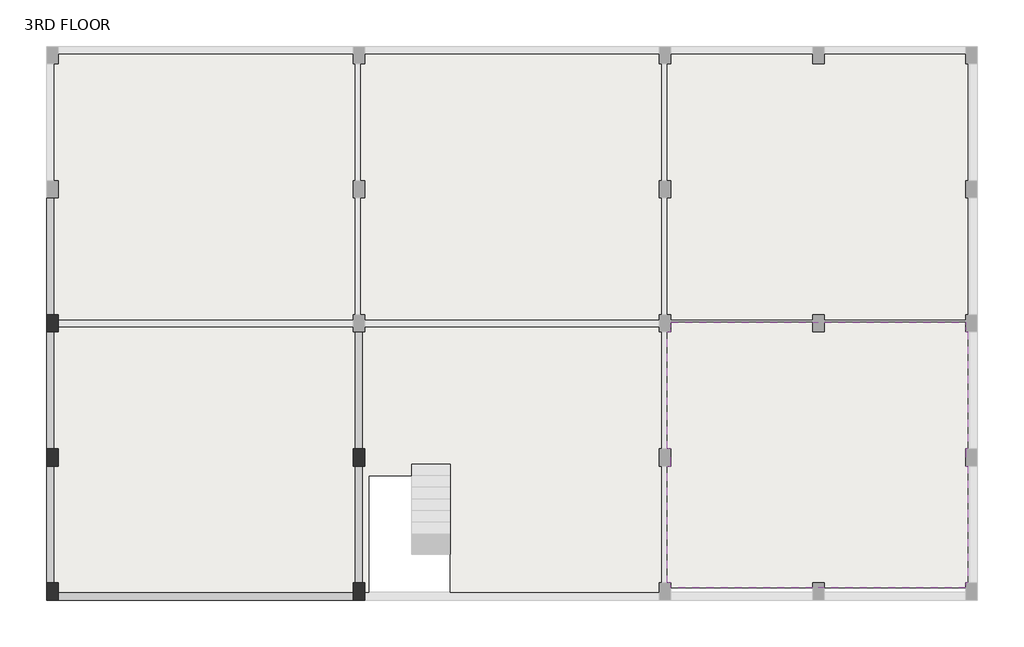
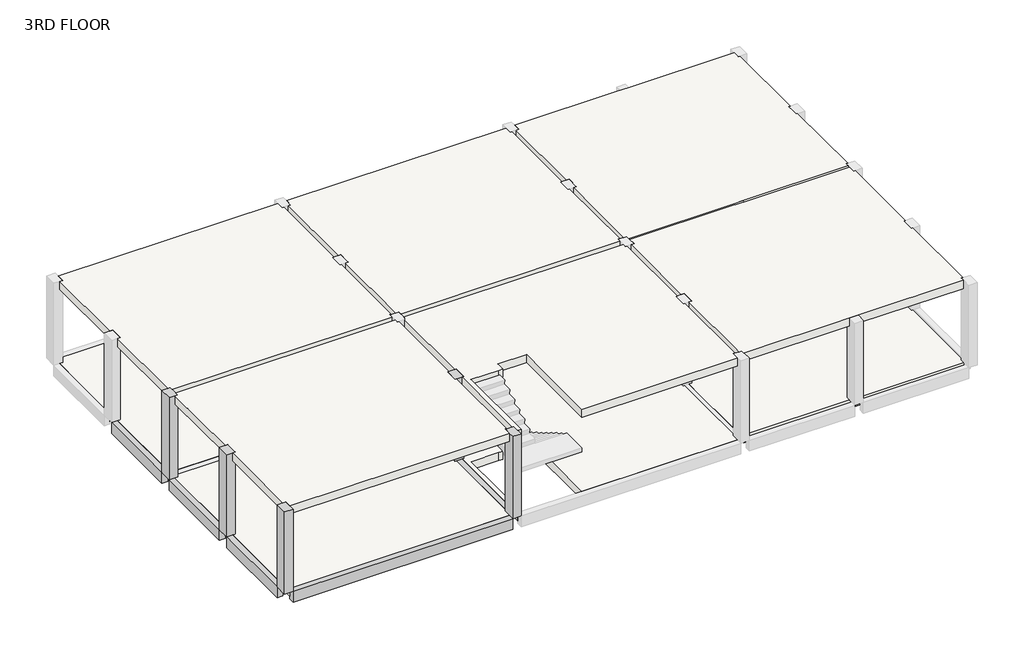
# One storey, part 1 of 2: 6 beams, 5 columns, 2 slabs.
"""IFC4 building model written with IfcOpenShell, lengths in millimetres."""

from ifc_helpers import new_model, si_unit, origin, place, context, project, spatial, faceted_brep, element, save

model = new_model("IFC4")

# Units and contexts
model_context = context("Model", 3, world=origin())
ifc_project = project(units=[si_unit("LENGTHUNIT", "METRE", prefix="MILLI")], contexts=[model_context])

# Site, building, storey
site = spatial("IfcSite", under=ifc_project)
building = spatial("IfcBuilding", under=site)
storey = spatial("IfcBuildingStorey", under=building, Name="3RD FLOOR", Elevation=9144.0)

# Beams
placement = place(None, origin())
element("IfcBeam", 1, ObjectType="M_Concrete-Rectangular Beam : 200MMX400MM", at=placement, inside=storey, context=model_context, shape_type="Brep", body=[
    faceted_brep([(-11680.6874017, 1747.7008557, 9144.0), (-11680.6874017, 1547.7008557, 9144.0), (-3980.6874017, 1547.7008557, 9144.0), (-3980.6874017, 1747.7008557, 9144.0), (-11680.6874017, 1747.7008557, 8744.0), (-11680.6874017, 1747.7008557, 8844.0), (-3980.6874017, 1747.7008557, 8844.0), (-3980.6874017, 1747.7008557, 8744.0), (-11680.6874017, 1547.7008557, 8744.0), (-3980.6874017, 1547.7008557, 8744.0)], [[[0, 1, 2, 3]], [[4, 5, 0, 3, 6, 7]], [[8, 4, 7, 9]], [[1, 8, 9, 2]], [[1, 0, 5, 4, 8]], [[2, 9, 7, 6, 3]]]),
])
element("IfcBeam", 2, ObjectType="M_Concrete-Rectangular Beam : 200MMX400MM", at=placement, inside=storey, context=model_context, shape_type="Brep", body=[
    faceted_brep([(-11980.6874017, 8997.7008557, 9144.0), (-11780.6874017, 8997.7008557, 9144.0), (-11780.6874017, 12047.7008557, 9144.0), (-11980.6874017, 12047.7008557, 9144.0), (-11980.6874017, 8997.7008557, 8744.0), (-11980.6874017, 12047.7008557, 8744.0), (-11780.6874017, 8997.7008557, 8744.0), (-11780.6874017, 12047.7008557, 8744.0), (-11780.6874017, 8997.7008557, 8844.0), (-11780.6874017, 12047.7008557, 8844.0)], [[[0, 1, 2, 3]], [[4, 0, 3, 5]], [[6, 4, 5, 7]], [[1, 8, 6, 7, 9, 2]], [[1, 0, 4, 6, 8]], [[2, 9, 7, 5, 3]]]),
])
element("IfcBeam", 3, ObjectType="M_Concrete-Rectangular Beam : 200MMX400MM", at=placement, inside=storey, context=model_context, shape_type="Brep", body=[
    faceted_brep([(-11980.6874017, 5497.7008557, 9144.0), (-11780.6874017, 5497.7008557, 9144.0), (-11780.6874017, 8547.7008557, 9144.0), (-11980.6874017, 8547.7008557, 9144.0), (-11980.6874017, 5497.7008557, 8744.0), (-11980.6874017, 8547.7008557, 8744.0), (-11780.6874017, 5497.7008557, 8744.0), (-11780.6874017, 8547.7008557, 8744.0), (-11780.6874017, 5497.7008557, 8844.0), (-11780.6874017, 8547.7008557, 8844.0)], [[[0, 1, 2, 3]], [[4, 0, 3, 5]], [[6, 4, 5, 7]], [[1, 8, 6, 7, 9, 2]], [[2, 9, 7, 5, 3]], [[1, 0, 4, 6, 8]]]),
])
element("IfcBeam", 4, ObjectType="M_Concrete-Rectangular Beam : 200MMX400MM", at=placement, inside=storey, context=model_context, shape_type="Brep", body=[
    faceted_brep([(-11980.6874017, 1997.7008557, 9144.0), (-11780.6874017, 1997.7008557, 9144.0), (-11780.6874017, 5047.7008557, 9144.0), (-11980.6874017, 5047.7008557, 9144.0), (-11980.6874017, 1997.7008557, 8744.0), (-11980.6874017, 5047.7008557, 8744.0), (-11780.6874017, 1997.7008557, 8744.0), (-11780.6874017, 5047.7008557, 8744.0), (-11780.6874017, 1997.7008557, 8844.0), (-11780.6874017, 5047.7008557, 8844.0)], [[[0, 1, 2, 3]], [[4, 0, 3, 5]], [[6, 4, 5, 7]], [[1, 8, 6, 7, 9, 2]], [[1, 0, 4, 6, 8]], [[2, 9, 7, 5, 3]]]),
])
element("IfcBeam", 5, ObjectType="M_Concrete-Rectangular Beam : 200MMX400MM", at=placement, inside=storey, context=model_context, shape_type="Brep", body=[
    faceted_brep([(-3930.6874017, 5047.7008557, 9144.0), (-3930.6874017, 1997.7008557, 9144.0), (-3730.6874017, 1997.7008557, 9144.0), (-3730.6874017, 5047.7008557, 9144.0), (-3730.6874017, 1997.7008557, 8844.0), (-3730.6874017, 1997.7008557, 8744.0), (-3730.6874017, 5047.7008557, 8744.0), (-3730.6874017, 5047.7008557, 8844.0), (-3930.6874017, 1997.7008557, 8744.0), (-3930.6874017, 5047.7008557, 8744.0), (-3930.6874017, 5047.7008557, 8844.0), (-3930.6874017, 1997.7008557, 8844.0)], [[[0, 1, 2, 3]], [[3, 2, 4, 5, 6, 7]], [[6, 5, 8, 9]], [[1, 0, 10, 9, 8, 11]], [[8, 5, 4, 2, 1, 11]], [[0, 3, 7, 6, 9, 10]]]),
])
element("IfcBeam", 6, ObjectType="M_Concrete-Rectangular Beam : 200MMX400MM", at=placement, inside=storey, context=model_context, shape_type="Brep", body=[
    faceted_brep([(-3930.6874017, 8547.7008557, 9144.0), (-3930.6874017, 5497.7008557, 9144.0), (-3730.6874017, 5497.7008557, 9144.0), (-3730.6874017, 8547.7008557, 9144.0), (-3730.6874017, 5497.7008557, 8844.0), (-3730.6874017, 5497.7008557, 8744.0), (-3730.6874017, 8547.7008557, 8744.0), (-3730.6874017, 8547.7008557, 8844.0), (-3930.6874017, 5497.7008557, 8744.0), (-3930.6874017, 8547.7008557, 8744.0), (-3930.6874017, 8547.7008557, 8844.0), (-3930.6874017, 5497.7008557, 8844.0)], [[[0, 1, 2, 3]], [[3, 2, 4, 5, 6, 7]], [[6, 5, 8, 9]], [[1, 0, 10, 9, 8, 11]], [[0, 3, 7, 6, 9, 10]], [[8, 5, 4, 2, 1, 11]]]),
])

# Columns
element("IfcColumn", 7, ObjectType="M_Concrete-Rectangular-Column : 300 x 450mm", at=placement, inside=storey, context=model_context, shape_type="Brep", body=[
    faceted_brep([(-11680.6874017, 8997.7008557, 9144.0), (-11680.6874017, 8547.7008557, 9144.0), (-11980.6874017, 8547.7008557, 9144.0), (-11980.6874017, 8997.7008557, 9144.0), (-11680.6874017, 8997.7008557, 11892.0), (-11680.6874017, 8997.7008557, 12192.0), (-11680.6874017, 8872.7008557, 12192.0), (-11680.6874017, 8672.7008557, 12192.0), (-11680.6874017, 8547.7008557, 12192.0), (-11680.6874017, 8547.7008557, 11892.0), (-11780.6874017, 8547.7008557, 12192.0), (-11980.6874017, 8547.7008557, 12192.0), (-11980.6874017, 8997.7008557, 12192.0), (-11780.6874017, 8997.7008557, 12192.0)], [[[0, 1, 2, 3]], [[1, 0, 4, 5, 6, 7, 8, 9]], [[2, 1, 9, 8, 10, 11]], [[3, 2, 11, 12]], [[0, 3, 12, 13, 5, 4]], [[12, 11, 10, 8, 7, 6, 5, 13]]]),
])
element("IfcColumn", 8, ObjectType="M_Concrete-Rectangular-Column : 300 x 450mm", at=placement, inside=storey, context=model_context, shape_type="Brep", body=[
    faceted_brep([(-11680.6874017, 1997.7008557, 9144.0), (-11680.6874017, 1547.7008557, 9144.0), (-11980.6874017, 1547.7008557, 9144.0), (-11980.6874017, 1997.7008557, 9144.0), (-11680.6874017, 1997.7008557, 11892.0), (-11680.6874017, 1997.7008557, 12192.0), (-11680.6874017, 1747.7008557, 12192.0), (-11680.6874017, 1547.7008557, 12192.0), (-11980.6874017, 1547.7008557, 12192.0), (-11980.6874017, 1997.7008557, 12192.0), (-11780.6874017, 1997.7008557, 12192.0)], [[[0, 1, 2, 3]], [[1, 0, 4, 5, 6, 7]], [[2, 1, 7, 8]], [[3, 2, 8, 9]], [[0, 3, 9, 10, 5, 4]], [[8, 7, 6, 5, 10, 9]]]),
])
element("IfcColumn", 9, ObjectType="M_Concrete-Rectangular-Column : 300 x 450mm", at=placement, inside=storey, context=model_context, shape_type="Brep", body=[
    faceted_brep([(-3680.6874017, 5497.7008557, 9144.0), (-3680.6874017, 5047.7008557, 9144.0), (-3980.6874017, 5047.7008557, 9144.0), (-3980.6874017, 5497.7008557, 9144.0), (-3680.6874017, 5497.7008557, 11892.0), (-3680.6874017, 5497.7008557, 12192.0), (-3680.6874017, 5047.7008557, 12192.0), (-3680.6874017, 5047.7008557, 11892.0), (-3730.6874017, 5047.7008557, 12192.0), (-3930.6874017, 5047.7008557, 12192.0), (-3980.6874017, 5047.7008557, 12192.0), (-3980.6874017, 5047.7008557, 11892.0), (-3980.6874017, 5497.7008557, 12192.0), (-3980.6874017, 5497.7008557, 11892.0), (-3930.6874017, 5497.7008557, 12192.0), (-3730.6874017, 5497.7008557, 12192.0)], [[[0, 1, 2, 3]], [[1, 0, 4, 5, 6, 7]], [[2, 1, 7, 6, 8, 9, 10, 11]], [[3, 2, 11, 10, 12, 13]], [[0, 3, 13, 12, 14, 15, 5, 4]], [[6, 5, 15, 14, 12, 10, 9, 8]]]),
])
element("IfcColumn", 10, ObjectType="M_Concrete-Rectangular-Column : 300 x 450mm", at=placement, inside=storey, context=model_context, shape_type="Brep", body=[
    faceted_brep([(-3680.6874017, 1997.7008557, 9144.0), (-3680.6874017, 1547.7008557, 9144.0), (-3980.6874017, 1547.7008557, 9144.0), (-3980.6874017, 1997.7008557, 9144.0), (-3680.6874017, 1997.7008557, 11892.0), (-3680.6874017, 1997.7008557, 12192.0), (-3680.6874017, 1747.7008557, 12192.0), (-3680.6874017, 1547.7008557, 12192.0), (-3980.6874017, 1547.7008557, 12192.0), (-3980.6874017, 1747.7008557, 12192.0), (-3980.6874017, 1997.7008557, 12192.0), (-3980.6874017, 1997.7008557, 11892.0), (-3930.6874017, 1997.7008557, 12192.0), (-3730.6874017, 1997.7008557, 12192.0)], [[[0, 1, 2, 3]], [[1, 0, 4, 5, 6, 7]], [[2, 1, 7, 8]], [[3, 2, 8, 9, 10, 11]], [[0, 3, 11, 10, 12, 13, 5, 4]], [[8, 7, 6, 5, 13, 12, 10, 9]]]),
])
element("IfcColumn", 11, ObjectType="M_Concrete-Rectangular-Column : 300 x 450mm", at=placement, inside=storey, context=model_context, shape_type="Brep", body=[
    faceted_brep([(-11680.6874017, 5497.7008557, 9144.0), (-11680.6874017, 5047.7008557, 9144.0), (-11980.6874017, 5047.7008557, 9144.0), (-11980.6874017, 5497.7008557, 9144.0), (-11680.6874017, 5497.7008557, 11892.0), (-11680.6874017, 5497.7008557, 12192.0), (-11680.6874017, 5047.7008557, 12192.0), (-11680.6874017, 5047.7008557, 11892.0), (-11780.6874017, 5047.7008557, 12192.0), (-11980.6874017, 5047.7008557, 12192.0), (-11980.6874017, 5497.7008557, 12192.0), (-11780.6874017, 5497.7008557, 12192.0)], [[[0, 1, 2, 3]], [[1, 0, 4, 5, 6, 7]], [[2, 1, 7, 6, 8, 9]], [[3, 2, 9, 10]], [[0, 3, 10, 11, 5, 4]], [[6, 5, 11, 10, 9, 8]]]),
])

# Slabs
element("IfcSlab", 12, ObjectType="Generic 300mm", at=placement, inside=storey, context=model_context, shape_type="Brep", body=[
    faceted_brep([(-11680.6874017, 15547.7008557, 8844.0), (-11680.6874017, 15797.7008557, 8844.0), (-3980.6874017, 15797.7008557, 8844.0), (-3980.6874017, 15547.7008557, 8844.0), (-3930.6874017, 15547.7008557, 8844.0), (-3930.6874017, 12497.7008557, 8844.0), (-3980.6874017, 12497.7008557, 8844.0), (-3980.6874017, 12047.7008557, 8844.0), (-3930.6874017, 12047.7008557, 8844.0), (-3930.6874017, 8997.7008557, 8844.0), (-3980.6874017, 8997.7008557, 8844.0), (-3980.6874017, 8872.7008557, 8844.0), (-11680.6874017, 8872.7008557, 8844.0), (-11680.6874017, 8997.7008557, 8844.0), (-11780.6874017, 8997.7008557, 8844.0), (-11780.6874017, 12047.7008557, 8844.0), (-11680.6874017, 12047.7008557, 8844.0), (-11680.6874017, 12497.7008557, 8844.0), (-11780.6874017, 12497.7008557, 8844.0), (-11780.6874017, 15547.7008557, 8844.0), (-11680.6874017, 15797.7008557, 9144.0), (-11680.6874017, 15547.7008557, 9144.0), (-11780.6874017, 15547.7008557, 9144.0), (-11780.6874017, 12497.7008557, 9144.0), (-11680.6874017, 12497.7008557, 9144.0), (-11680.6874017, 12047.7008557, 9144.0), (-11780.6874017, 12047.7008557, 9144.0), (-11780.6874017, 8997.7008557, 9144.0), (-11680.6874017, 8997.7008557, 9144.0), (-11680.6874017, 8872.7008557, 9144.0), (-3980.6874017, 8872.7008557, 9144.0), (-3980.6874017, 8997.7008557, 9144.0), (-3930.6874017, 8997.7008557, 9144.0), (-3930.6874017, 12047.7008557, 9144.0), (-3980.6874017, 12047.7008557, 9144.0), (-3980.6874017, 12497.7008557, 9144.0), (-3930.6874017, 12497.7008557, 9144.0), (-3930.6874017, 15547.7008557, 9144.0), (-3980.6874017, 15547.7008557, 9144.0), (-3980.6874017, 15797.7008557, 9144.0)], [[[0, 1, 2, 3, 4, 5, 6, 7, 8, 9, 10, 11, 12, 13, 14, 15, 16, 17, 18, 19]], [[20, 21, 22, 23, 24, 25, 26, 27, 28, 29, 30, 31, 32, 33, 34, 35, 36, 37, 38, 39]], [[1, 0, 21, 20]], [[2, 1, 20, 39]], [[3, 2, 39, 38]], [[4, 3, 38, 37]], [[5, 4, 37, 36]], [[6, 5, 36, 35]], [[7, 6, 35, 34]], [[8, 7, 34, 33]], [[9, 8, 33, 32]], [[10, 9, 32, 31]], [[11, 10, 31, 30]], [[12, 11, 30, 29]], [[13, 12, 29, 28]], [[14, 13, 28, 27]], [[15, 14, 27, 26]], [[16, 15, 26, 25]], [[17, 16, 25, 24]], [[18, 17, 24, 23]], [[19, 18, 23, 22]], [[0, 19, 22, 21]]]),
    faceted_brep([(-3680.6874017, 15547.7008557, 8844.0), (-3680.6874017, 15797.7008557, 8844.0), (4019.3125983, 15797.7008557, 8844.0), (4019.3125983, 15547.7008557, 8844.0), (4069.3125983, 15547.7008557, 8844.0), (4069.3125983, 12497.7008557, 8844.0), (4019.3125983, 12497.7008557, 8844.0), (4019.3125983, 12047.7008557, 8844.0), (4069.3125983, 12047.7008557, 8844.0), (4069.3125983, 8997.7008557, 8844.0), (4019.3125983, 8997.7008557, 8844.0), (4019.3125983, 8872.7008557, 8844.0), (-3680.6874017, 8872.7008557, 8844.0), (-3680.6874017, 8997.7008557, 8844.0), (-3730.6874017, 8997.7008557, 8844.0), (-3780.6874017, 8997.7008557, 8844.0), (-3780.6874017, 12047.7008557, 8844.0), (-3730.6874017, 12047.7008557, 8844.0), (-3680.6874017, 12047.7008557, 8844.0), (-3680.6874017, 12497.7008557, 8844.0), (-3730.6874017, 12497.7008557, 8844.0), (-3780.6874017, 12497.7008557, 8844.0), (-3780.6874017, 15547.7008557, 8844.0), (-3730.6874017, 15547.7008557, 8844.0), (-3680.6874017, 15797.7008557, 9144.0), (-3680.6874017, 15547.7008557, 9144.0), (-3780.6874017, 15547.7008557, 9144.0), (-3780.6874017, 12497.7008557, 9144.0), (-3680.6874017, 12497.7008557, 9144.0), (-3680.6874017, 12047.7008557, 9144.0), (-3780.6874017, 12047.7008557, 9144.0), (-3780.6874017, 8997.7008557, 9144.0), (-3680.6874017, 8997.7008557, 9144.0), (-3680.6874017, 8872.7008557, 9144.0), (4019.3125983, 8872.7008557, 9144.0), (4019.3125983, 8997.7008557, 9144.0), (4069.3125983, 8997.7008557, 9144.0), (4069.3125983, 12047.7008557, 9144.0), (4019.3125983, 12047.7008557, 9144.0), (4019.3125983, 12497.7008557, 9144.0), (4069.3125983, 12497.7008557, 9144.0), (4069.3125983, 15547.7008557, 9144.0), (4019.3125983, 15547.7008557, 9144.0), (4019.3125983, 15797.7008557, 9144.0)], [[[0, 1, 2, 3, 4, 5, 6, 7, 8, 9, 10, 11, 12, 13, 14, 15, 16, 17, 18, 19, 20, 21, 22, 23]], [[24, 25, 26, 27, 28, 29, 30, 31, 32, 33, 34, 35, 36, 37, 38, 39, 40, 41, 42, 43]], [[1, 0, 25, 24]], [[2, 1, 24, 43]], [[3, 2, 43, 42]], [[4, 3, 42, 41]], [[5, 4, 41, 40]], [[6, 5, 40, 39]], [[7, 6, 39, 38]], [[8, 7, 38, 37]], [[9, 8, 37, 36]], [[10, 9, 36, 35]], [[11, 10, 35, 34]], [[12, 11, 34, 33]], [[13, 12, 33, 32]], [[15, 14, 13, 32, 31]], [[16, 15, 31, 30]], [[18, 17, 16, 30, 29]], [[19, 18, 29, 28]], [[21, 20, 19, 28, 27]], [[22, 21, 27, 26]], [[0, 23, 22, 26, 25]]]),
    faceted_brep([(4319.3125983, 15547.7008557, 8844.0), (4319.3125983, 15797.7008557, 8844.0), (8019.3125983, 15797.7008557, 8844.0), (8319.3125983, 15797.7008557, 8844.0), (12019.3125983, 15797.7008557, 8844.0), (12019.3125983, 15547.7008557, 8844.0), (12069.3125983, 15547.7008557, 8844.0), (12069.3125983, 12497.7008557, 8844.0), (12019.3125983, 12497.7008557, 8844.0), (12019.3125983, 12047.7008557, 8844.0), (12069.3125983, 12047.7008557, 8844.0), (12069.3125983, 8997.7008557, 8844.0), (12019.3125983, 8997.7008557, 8844.0), (12019.3125983, 8872.7008557, 8844.0), (8319.3125983, 8872.7008557, 8844.0), (8019.3125983, 8872.7008557, 8844.0), (4319.3125983, 8872.7008557, 8844.0), (4319.3125983, 8997.7008557, 8844.0), (4269.3125983, 8997.7008557, 8844.0), (4219.3125983, 8997.7008557, 8844.0), (4219.3125983, 12047.7008557, 8844.0), (4269.3125983, 12047.7008557, 8844.0), (4319.3125983, 12047.7008557, 8844.0), (4319.3125983, 12497.7008557, 8844.0), (4269.3125983, 12497.7008557, 8844.0), (4219.3125983, 12497.7008557, 8844.0), (4219.3125983, 15547.7008557, 8844.0), (4269.3125983, 15547.7008557, 8844.0), (4319.3125983, 15797.7008557, 9144.0), (4319.3125983, 15547.7008557, 9144.0), (4219.3125983, 15547.7008557, 9144.0), (4219.3125983, 12497.7008557, 9144.0), (4319.3125983, 12497.7008557, 9144.0), (4319.3125983, 12047.7008557, 9144.0), (4219.3125983, 12047.7008557, 9144.0), (4219.3125983, 8997.7008557, 9144.0), (4319.3125983, 8997.7008557, 9144.0), (4319.3125983, 8872.7008557, 9144.0), (8019.3125983, 8872.7008557, 9144.0), (8319.3125983, 8872.7008557, 9144.0), (12019.3125983, 8872.7008557, 9144.0), (12019.3125983, 8997.7008557, 9144.0), (12069.3125983, 8997.7008557, 9144.0), (12069.3125983, 12047.7008557, 9144.0), (12019.3125983, 12047.7008557, 9144.0), (12019.3125983, 12497.7008557, 9144.0), (12069.3125983, 12497.7008557, 9144.0), (12069.3125983, 15547.7008557, 9144.0), (12019.3125983, 15547.7008557, 9144.0), (12019.3125983, 15797.7008557, 9144.0), (8319.3125983, 15797.7008557, 9144.0), (8019.3125983, 15797.7008557, 9144.0)], [[[0, 1, 2, 3, 4, 5, 6, 7, 8, 9, 10, 11, 12, 13, 14, 15, 16, 17, 18, 19, 20, 21, 22, 23, 24, 25, 26, 27]], [[28, 29, 30, 31, 32, 33, 34, 35, 36, 37, 38, 39, 40, 41, 42, 43, 44, 45, 46, 47, 48, 49, 50, 51]], [[1, 0, 29, 28]], [[4, 3, 2, 1, 28, 51, 50, 49]], [[5, 4, 49, 48]], [[6, 5, 48, 47]], [[7, 6, 47, 46]], [[8, 7, 46, 45]], [[9, 8, 45, 44]], [[10, 9, 44, 43]], [[11, 10, 43, 42]], [[12, 11, 42, 41]], [[13, 12, 41, 40]], [[16, 15, 14, 13, 40, 39, 38, 37]], [[17, 16, 37, 36]], [[19, 18, 17, 36, 35]], [[20, 19, 35, 34]], [[22, 21, 20, 34, 33]], [[23, 22, 33, 32]], [[25, 24, 23, 32, 31]], [[26, 25, 31, 30]], [[0, 27, 26, 30, 29]]]),
    faceted_brep([(-3680.6874017, 8547.7008557, 8844.0), (-3680.6874017, 8672.7008557, 8844.0), (4019.3125983, 8672.7008557, 8844.0), (4019.3125983, 8547.7008557, 8844.0), (4069.3125983, 8547.7008557, 8844.0), (4069.3125983, 5497.7008557, 8844.0), (4019.3125983, 5497.7008557, 8844.0), (4019.3125983, 5047.7008557, 8844.0), (4069.3125983, 5047.7008557, 8844.0), (4069.3125983, 1997.7008557, 8844.0), (4019.3125983, 1997.7008557, 8844.0), (4019.3125983, 1747.7008557, 8844.0), (-1437.0874017, 1747.7008557, 8844.0), (-1437.0874017, 5100.5008557, 8844.0), (-2453.0874017, 5100.5008557, 8844.0), (-2453.0874017, 4795.7008557, 8844.0), (-2593.0874017, 4795.7008557, 8844.0), (-3570.6874017, 4795.7008557, 8844.0), (-3570.6874017, 1747.7008557, 8844.0), (-3680.6874017, 1747.7008557, 8844.0), (-3680.6874017, 1997.7008557, 8844.0), (-3730.6874017, 1997.7008557, 8844.0), (-3730.6874017, 5047.7008557, 8844.0), (-3680.6874017, 5047.7008557, 8844.0), (-3680.6874017, 5497.7008557, 8844.0), (-3730.6874017, 5497.7008557, 8844.0), (-3730.6874017, 8547.7008557, 8844.0), (-3680.6874017, 8672.7008557, 9144.0), (-3680.6874017, 8547.7008557, 9144.0), (-3730.6874017, 8547.7008557, 9144.0), (-3730.6874017, 5497.7008557, 9144.0), (-3680.6874017, 5497.7008557, 9144.0), (-3680.6874017, 5047.7008557, 9144.0), (-3730.6874017, 5047.7008557, 9144.0), (-3730.6874017, 1997.7008557, 9144.0), (-3680.6874017, 1997.7008557, 9144.0), (-3680.6874017, 1747.7008557, 9144.0), (-3570.6874017, 1747.7008557, 9144.0), (-3570.6874017, 4795.7008557, 9144.0), (-2593.0874017, 4795.7008557, 9144.0), (-2453.0874017, 4795.7008557, 9144.0), (-2453.0874017, 5100.5008557, 9144.0), (-1437.0874017, 5100.5008557, 9144.0), (-1437.0874017, 1747.7008557, 9144.0), (4019.3125983, 1747.7008557, 9144.0), (4019.3125983, 1997.7008557, 9144.0), (4069.3125983, 1997.7008557, 9144.0), (4069.3125983, 5047.7008557, 9144.0), (4019.3125983, 5047.7008557, 9144.0), (4019.3125983, 5497.7008557, 9144.0), (4069.3125983, 5497.7008557, 9144.0), (4069.3125983, 8547.7008557, 9144.0), (4019.3125983, 8547.7008557, 9144.0), (4019.3125983, 8672.7008557, 9144.0)], [[[0, 1, 2, 3, 4, 5, 6, 7, 8, 9, 10, 11, 12, 13, 14, 15, 16, 17, 18, 19, 20, 21, 22, 23, 24, 25, 26]], [[27, 28, 29, 30, 31, 32, 33, 34, 35, 36, 37, 38, 39, 40, 41, 42, 43, 44, 45, 46, 47, 48, 49, 50, 51, 52, 53]], [[1, 0, 28, 27]], [[2, 1, 27, 53]], [[3, 2, 53, 52]], [[4, 3, 52, 51]], [[5, 4, 51, 50]], [[6, 5, 50, 49]], [[7, 6, 49, 48]], [[8, 7, 48, 47]], [[9, 8, 47, 46]], [[10, 9, 46, 45]], [[11, 10, 45, 44]], [[11, 44, 43, 12]], [[36, 19, 18, 37]], [[20, 19, 36, 35]], [[21, 20, 35, 34]], [[22, 21, 34, 33]], [[23, 22, 33, 32]], [[24, 23, 32, 31]], [[25, 24, 31, 30]], [[26, 25, 30, 29]], [[0, 26, 29, 28]], [[42, 13, 12, 43]], [[13, 42, 41, 14]], [[14, 41, 40, 15]], [[15, 40, 39, 16]], [[16, 39, 38, 17]], [[17, 38, 37, 18]]]),
    faceted_brep([(-3980.6874017, 1747.7008557, 8844.0), (-11680.6874017, 1747.7008557, 8844.0), (-11680.6874017, 1997.7008557, 8844.0), (-11780.6874017, 1997.7008557, 8844.0), (-11780.6874017, 5047.7008557, 8844.0), (-11680.6874017, 5047.7008557, 8844.0), (-11680.6874017, 5497.7008557, 8844.0), (-11780.6874017, 5497.7008557, 8844.0), (-11780.6874017, 8547.7008557, 8844.0), (-11680.6874017, 8547.7008557, 8844.0), (-11680.6874017, 8672.7008557, 8844.0), (-3980.6874017, 8672.7008557, 8844.0), (-3980.6874017, 8547.7008557, 8844.0), (-3930.6874017, 8547.7008557, 8844.0), (-3930.6874017, 5497.7008557, 8844.0), (-3980.6874017, 5497.7008557, 8844.0), (-3980.6874017, 5047.7008557, 8844.0), (-3930.6874017, 5047.7008557, 8844.0), (-3930.6874017, 1997.7008557, 8844.0), (-3980.6874017, 1997.7008557, 8844.0), (-11680.6874017, 1747.7008557, 9144.0), (-3980.6874017, 1747.7008557, 9144.0), (-3980.6874017, 1997.7008557, 9144.0), (-3930.6874017, 1997.7008557, 9144.0), (-3930.6874017, 5047.7008557, 9144.0), (-3980.6874017, 5047.7008557, 9144.0), (-3980.6874017, 5497.7008557, 9144.0), (-3930.6874017, 5497.7008557, 9144.0), (-3930.6874017, 8547.7008557, 9144.0), (-3980.6874017, 8547.7008557, 9144.0), (-3980.6874017, 8672.7008557, 9144.0), (-11680.6874017, 8672.7008557, 9144.0), (-11680.6874017, 8547.7008557, 9144.0), (-11780.6874017, 8547.7008557, 9144.0), (-11780.6874017, 5497.7008557, 9144.0), (-11680.6874017, 5497.7008557, 9144.0), (-11680.6874017, 5047.7008557, 9144.0), (-11780.6874017, 5047.7008557, 9144.0), (-11780.6874017, 1997.7008557, 9144.0), (-11680.6874017, 1997.7008557, 9144.0)], [[[0, 1, 2, 3, 4, 5, 6, 7, 8, 9, 10, 11, 12, 13, 14, 15, 16, 17, 18, 19]], [[20, 21, 22, 23, 24, 25, 26, 27, 28, 29, 30, 31, 32, 33, 34, 35, 36, 37, 38, 39]], [[1, 0, 21, 20]], [[2, 1, 20, 39]], [[3, 2, 39, 38]], [[4, 3, 38, 37]], [[5, 4, 37, 36]], [[6, 5, 36, 35]], [[7, 6, 35, 34]], [[8, 7, 34, 33]], [[9, 8, 33, 32]], [[10, 9, 32, 31]], [[11, 10, 31, 30]], [[12, 11, 30, 29]], [[13, 12, 29, 28]], [[14, 13, 28, 27]], [[15, 14, 27, 26]], [[16, 15, 26, 25]], [[17, 16, 25, 24]], [[18, 17, 24, 23]], [[19, 18, 23, 22]], [[0, 19, 22, 21]]]),
    faceted_brep([(4319.3125983, 8547.7008557, 8844.0), (4319.3125983, 8672.7008557, 8844.0), (4319.3125983, 8797.7008557, 8844.0), (8019.3125983, 8797.7008557, 8844.0), (8319.3125983, 8797.7008557, 8844.0), (12019.3125983, 8797.7008557, 8844.0), (12019.3125983, 8672.7008557, 8844.0), (12019.3125983, 8547.7008557, 8844.0), (12069.3125983, 8547.7008557, 8844.0), (12069.3125983, 5497.7008557, 8844.0), (12019.3125983, 5497.7008557, 8844.0), (12019.3125983, 5047.7008557, 8844.0), (12069.3125983, 5047.7008557, 8844.0), (12069.3125983, 1997.7008557, 8844.0), (12019.3125983, 1997.7008557, 8844.0), (12019.3125983, 1872.7008557, 8844.0), (8319.3125983, 1872.7008557, 8844.0), (8019.3125983, 1872.7008557, 8844.0), (4319.3125983, 1872.7008557, 8844.0), (4319.3125983, 1997.7008557, 8844.0), (4269.3125983, 1997.7008557, 8844.0), (4219.3125983, 1997.7008557, 8844.0), (4219.3125983, 5047.7008557, 8844.0), (4269.3125983, 5047.7008557, 8844.0), (4319.3125983, 5047.7008557, 8844.0), (4319.3125983, 5497.7008557, 8844.0), (4269.3125983, 5497.7008557, 8844.0), (4219.3125983, 5497.7008557, 8844.0), (4219.3125983, 8547.7008557, 8844.0), (4269.3125983, 8547.7008557, 8844.0), (4319.3125983, 8797.7008557, 9144.0), (4319.3125983, 8547.7008557, 9144.0), (4219.3125983, 8547.7008557, 9144.0), (4219.3125983, 5497.7008557, 9144.0), (4319.3125983, 5497.7008557, 9144.0), (4319.3125983, 5047.7008557, 9144.0), (4219.3125983, 5047.7008557, 9144.0), (4219.3125983, 1997.7008557, 9144.0), (4319.3125983, 1997.7008557, 9144.0), (4319.3125983, 1872.7008557, 9144.0), (8019.3125983, 1872.7008557, 9144.0), (8319.3125983, 1872.7008557, 9144.0), (12019.3125983, 1872.7008557, 9144.0), (12019.3125983, 1997.7008557, 9144.0), (12069.3125983, 1997.7008557, 9144.0), (12069.3125983, 5047.7008557, 9144.0), (12019.3125983, 5047.7008557, 9144.0), (12019.3125983, 5497.7008557, 9144.0), (12069.3125983, 5497.7008557, 9144.0), (12069.3125983, 8547.7008557, 9144.0), (12019.3125983, 8547.7008557, 9144.0), (12019.3125983, 8797.7008557, 9144.0), (8319.3125983, 8797.7008557, 9144.0), (8019.3125983, 8797.7008557, 9144.0)], [[[0, 1, 2, 3, 4, 5, 6, 7, 8, 9, 10, 11, 12, 13, 14, 15, 16, 17, 18, 19, 20, 21, 22, 23, 24, 25, 26, 27, 28, 29]], [[30, 31, 32, 33, 34, 35, 36, 37, 38, 39, 40, 41, 42, 43, 44, 45, 46, 47, 48, 49, 50, 51, 52, 53]], [[2, 1, 0, 31, 30]], [[5, 4, 3, 2, 30, 53, 52, 51]], [[7, 6, 5, 51, 50]], [[8, 7, 50, 49]], [[9, 8, 49, 48]], [[10, 9, 48, 47]], [[11, 10, 47, 46]], [[12, 11, 46, 45]], [[13, 12, 45, 44]], [[14, 13, 44, 43]], [[15, 14, 43, 42]], [[18, 17, 16, 15, 42, 41, 40, 39]], [[19, 18, 39, 38]], [[21, 20, 19, 38, 37]], [[22, 21, 37, 36]], [[24, 23, 22, 36, 35]], [[25, 24, 35, 34]], [[27, 26, 25, 34, 33]], [[28, 27, 33, 32]], [[0, 29, 28, 32, 31]]]),
])
element("IfcSlab", 13, ObjectType="Generic 300mm", at=placement, inside=storey, context=model_context, shape_type="Brep", body=[
    faceted_brep([(-11680.6874017, 15547.7008557, 11892.0), (-11680.6874017, 15797.7008557, 11892.0), (-3980.6874017, 15797.7008557, 11892.0), (-3980.6874017, 15547.7008557, 11892.0), (-3930.6874017, 15547.7008557, 11892.0), (-3930.6874017, 12497.7008557, 11892.0), (-3980.6874017, 12497.7008557, 11892.0), (-3980.6874017, 12047.7008557, 11892.0), (-3930.6874017, 12047.7008557, 11892.0), (-3930.6874017, 8997.7008557, 11892.0), (-3980.6874017, 8997.7008557, 11892.0), (-3980.6874017, 8872.7008557, 11892.0), (-11680.6874017, 8872.7008557, 11892.0), (-11680.6874017, 8997.7008557, 11892.0), (-11780.6874017, 8997.7008557, 11892.0), (-11780.6874017, 12047.7008557, 11892.0), (-11680.6874017, 12047.7008557, 11892.0), (-11680.6874017, 12497.7008557, 11892.0), (-11780.6874017, 12497.7008557, 11892.0), (-11780.6874017, 15547.7008557, 11892.0), (-11680.6874017, 15797.7008557, 12192.0), (-11680.6874017, 15547.7008557, 12192.0), (-11780.6874017, 15547.7008557, 12192.0), (-11780.6874017, 12497.7008557, 12192.0), (-11680.6874017, 12497.7008557, 12192.0), (-11680.6874017, 12047.7008557, 12192.0), (-11780.6874017, 12047.7008557, 12192.0), (-11780.6874017, 8997.7008557, 12192.0), (-11680.6874017, 8997.7008557, 12192.0), (-11680.6874017, 8872.7008557, 12192.0), (-3980.6874017, 8872.7008557, 12192.0), (-3980.6874017, 8997.7008557, 12192.0), (-3930.6874017, 8997.7008557, 12192.0), (-3930.6874017, 12047.7008557, 12192.0), (-3980.6874017, 12047.7008557, 12192.0), (-3980.6874017, 12497.7008557, 12192.0), (-3930.6874017, 12497.7008557, 12192.0), (-3930.6874017, 15547.7008557, 12192.0), (-3980.6874017, 15547.7008557, 12192.0), (-3980.6874017, 15797.7008557, 12192.0)], [[[0, 1, 2, 3, 4, 5, 6, 7, 8, 9, 10, 11, 12, 13, 14, 15, 16, 17, 18, 19]], [[20, 21, 22, 23, 24, 25, 26, 27, 28, 29, 30, 31, 32, 33, 34, 35, 36, 37, 38, 39]], [[1, 0, 21, 20]], [[2, 1, 20, 39]], [[3, 2, 39, 38]], [[4, 3, 38, 37]], [[5, 4, 37, 36]], [[6, 5, 36, 35]], [[7, 6, 35, 34]], [[8, 7, 34, 33]], [[9, 8, 33, 32]], [[10, 9, 32, 31]], [[11, 10, 31, 30]], [[12, 11, 30, 29]], [[13, 12, 29, 28]], [[14, 13, 28, 27]], [[15, 14, 27, 26]], [[16, 15, 26, 25]], [[17, 16, 25, 24]], [[18, 17, 24, 23]], [[19, 18, 23, 22]], [[0, 19, 22, 21]]]),
    faceted_brep([(-3680.6874017, 15547.7008557, 11892.0), (-3680.6874017, 15797.7008557, 11892.0), (4019.3125983, 15797.7008557, 11892.0), (4019.3125983, 15547.7008557, 11892.0), (4069.3125983, 15547.7008557, 11892.0), (4069.3125983, 12497.7008557, 11892.0), (4019.3125983, 12497.7008557, 11892.0), (4019.3125983, 12047.7008557, 11892.0), (4069.3125983, 12047.7008557, 11892.0), (4069.3125983, 8997.7008557, 11892.0), (4019.3125983, 8997.7008557, 11892.0), (4019.3125983, 8872.7008557, 11892.0), (-3680.6874017, 8872.7008557, 11892.0), (-3680.6874017, 8997.7008557, 11892.0), (-3730.6874017, 8997.7008557, 11892.0), (-3780.6874017, 8997.7008557, 11892.0), (-3780.6874017, 12047.7008557, 11892.0), (-3730.6874017, 12047.7008557, 11892.0), (-3680.6874017, 12047.7008557, 11892.0), (-3680.6874017, 12497.7008557, 11892.0), (-3730.6874017, 12497.7008557, 11892.0), (-3780.6874017, 12497.7008557, 11892.0), (-3780.6874017, 15547.7008557, 11892.0), (-3730.6874017, 15547.7008557, 11892.0), (-3680.6874017, 15797.7008557, 12192.0), (-3680.6874017, 15547.7008557, 12192.0), (-3780.6874017, 15547.7008557, 12192.0), (-3780.6874017, 12497.7008557, 12192.0), (-3680.6874017, 12497.7008557, 12192.0), (-3680.6874017, 12047.7008557, 12192.0), (-3780.6874017, 12047.7008557, 12192.0), (-3780.6874017, 8997.7008557, 12192.0), (-3680.6874017, 8997.7008557, 12192.0), (-3680.6874017, 8872.7008557, 12192.0), (4019.3125983, 8872.7008557, 12192.0), (4019.3125983, 8997.7008557, 12192.0), (4069.3125983, 8997.7008557, 12192.0), (4069.3125983, 12047.7008557, 12192.0), (4019.3125983, 12047.7008557, 12192.0), (4019.3125983, 12497.7008557, 12192.0), (4069.3125983, 12497.7008557, 12192.0), (4069.3125983, 15547.7008557, 12192.0), (4019.3125983, 15547.7008557, 12192.0), (4019.3125983, 15797.7008557, 12192.0)], [[[0, 1, 2, 3, 4, 5, 6, 7, 8, 9, 10, 11, 12, 13, 14, 15, 16, 17, 18, 19, 20, 21, 22, 23]], [[24, 25, 26, 27, 28, 29, 30, 31, 32, 33, 34, 35, 36, 37, 38, 39, 40, 41, 42, 43]], [[1, 0, 25, 24]], [[2, 1, 24, 43]], [[3, 2, 43, 42]], [[4, 3, 42, 41]], [[5, 4, 41, 40]], [[6, 5, 40, 39]], [[7, 6, 39, 38]], [[8, 7, 38, 37]], [[9, 8, 37, 36]], [[10, 9, 36, 35]], [[11, 10, 35, 34]], [[12, 11, 34, 33]], [[13, 12, 33, 32]], [[15, 14, 13, 32, 31]], [[16, 15, 31, 30]], [[18, 17, 16, 30, 29]], [[19, 18, 29, 28]], [[21, 20, 19, 28, 27]], [[22, 21, 27, 26]], [[0, 23, 22, 26, 25]]]),
    faceted_brep([(4319.3125983, 15547.7008557, 11892.0), (4319.3125983, 15797.7008557, 11892.0), (8019.3125983, 15797.7008557, 11892.0), (8319.3125983, 15797.7008557, 11892.0), (12019.3125983, 15797.7008557, 11892.0), (12019.3125983, 15547.7008557, 11892.0), (12069.3125983, 15547.7008557, 11892.0), (12069.3125983, 12497.7008557, 11892.0), (12019.3125983, 12497.7008557, 11892.0), (12019.3125983, 12047.7008557, 11892.0), (12069.3125983, 12047.7008557, 11892.0), (12069.3125983, 8997.7008557, 11892.0), (12019.3125983, 8997.7008557, 11892.0), (12019.3125983, 8872.7008557, 11892.0), (8319.3125983, 8872.7008557, 11892.0), (8019.3125983, 8872.7008557, 11892.0), (4319.3125983, 8872.7008557, 11892.0), (4319.3125983, 8997.7008557, 11892.0), (4269.3125983, 8997.7008557, 11892.0), (4219.3125983, 8997.7008557, 11892.0), (4219.3125983, 12047.7008557, 11892.0), (4269.3125983, 12047.7008557, 11892.0), (4319.3125983, 12047.7008557, 11892.0), (4319.3125983, 12497.7008557, 11892.0), (4269.3125983, 12497.7008557, 11892.0), (4219.3125983, 12497.7008557, 11892.0), (4219.3125983, 15547.7008557, 11892.0), (4269.3125983, 15547.7008557, 11892.0), (4319.3125983, 15797.7008557, 12192.0), (4319.3125983, 15547.7008557, 12192.0), (4219.3125983, 15547.7008557, 12192.0), (4219.3125983, 12497.7008557, 12192.0), (4319.3125983, 12497.7008557, 12192.0), (4319.3125983, 12047.7008557, 12192.0), (4219.3125983, 12047.7008557, 12192.0), (4219.3125983, 8997.7008557, 12192.0), (4319.3125983, 8997.7008557, 12192.0), (4319.3125983, 8872.7008557, 12192.0), (8019.3125983, 8872.7008557, 12192.0), (8319.3125983, 8872.7008557, 12192.0), (12019.3125983, 8872.7008557, 12192.0), (12019.3125983, 8997.7008557, 12192.0), (12069.3125983, 8997.7008557, 12192.0), (12069.3125983, 12047.7008557, 12192.0), (12019.3125983, 12047.7008557, 12192.0), (12019.3125983, 12497.7008557, 12192.0), (12069.3125983, 12497.7008557, 12192.0), (12069.3125983, 15547.7008557, 12192.0), (12019.3125983, 15547.7008557, 12192.0), (12019.3125983, 15797.7008557, 12192.0), (8319.3125983, 15797.7008557, 12192.0), (8019.3125983, 15797.7008557, 12192.0)], [[[0, 1, 2, 3, 4, 5, 6, 7, 8, 9, 10, 11, 12, 13, 14, 15, 16, 17, 18, 19, 20, 21, 22, 23, 24, 25, 26, 27]], [[28, 29, 30, 31, 32, 33, 34, 35, 36, 37, 38, 39, 40, 41, 42, 43, 44, 45, 46, 47, 48, 49, 50, 51]], [[1, 0, 29, 28]], [[4, 3, 2, 1, 28, 51, 50, 49]], [[5, 4, 49, 48]], [[6, 5, 48, 47]], [[7, 6, 47, 46]], [[8, 7, 46, 45]], [[9, 8, 45, 44]], [[10, 9, 44, 43]], [[11, 10, 43, 42]], [[12, 11, 42, 41]], [[13, 12, 41, 40]], [[16, 15, 14, 13, 40, 39, 38, 37]], [[17, 16, 37, 36]], [[19, 18, 17, 36, 35]], [[20, 19, 35, 34]], [[22, 21, 20, 34, 33]], [[23, 22, 33, 32]], [[25, 24, 23, 32, 31]], [[26, 25, 31, 30]], [[0, 27, 26, 30, 29]]]),
    faceted_brep([(-3680.6874017, 8547.7008557, 11892.0), (-3680.6874017, 8672.7008557, 11892.0), (4019.3125983, 8672.7008557, 11892.0), (4019.3125983, 8547.7008557, 11892.0), (4069.3125983, 8547.7008557, 11892.0), (4069.3125983, 5497.7008557, 11892.0), (4019.3125983, 5497.7008557, 11892.0), (4019.3125983, 5047.7008557, 11892.0), (4069.3125983, 5047.7008557, 11892.0), (4069.3125983, 1997.7008557, 11892.0), (4019.3125983, 1997.7008557, 11892.0), (4019.3125983, 1747.7008557, 11892.0), (-1437.0874017, 1747.7008557, 11892.0), (-1437.0874017, 5100.5008557, 11892.0), (-2453.0874017, 5100.5008557, 11892.0), (-2453.0874017, 4795.7008557, 11892.0), (-2593.0874017, 4795.7008557, 11892.0), (-3570.6874017, 4795.7008557, 11892.0), (-3570.6874017, 1747.7008557, 11892.0), (-3680.6874017, 1747.7008557, 11892.0), (-3680.6874017, 1997.7008557, 11892.0), (-3730.6874017, 1997.7008557, 11892.0), (-3730.6874017, 5047.7008557, 11892.0), (-3680.6874017, 5047.7008557, 11892.0), (-3680.6874017, 5497.7008557, 11892.0), (-3730.6874017, 5497.7008557, 11892.0), (-3730.6874017, 8547.7008557, 11892.0), (-3680.6874017, 8672.7008557, 12192.0), (-3680.6874017, 8547.7008557, 12192.0), (-3730.6874017, 8547.7008557, 12192.0), (-3730.6874017, 5497.7008557, 12192.0), (-3680.6874017, 5497.7008557, 12192.0), (-3680.6874017, 5047.7008557, 12192.0), (-3730.6874017, 5047.7008557, 12192.0), (-3730.6874017, 1997.7008557, 12192.0), (-3680.6874017, 1997.7008557, 12192.0), (-3680.6874017, 1747.7008557, 12192.0), (-3570.6874017, 1747.7008557, 12192.0), (-3570.6874017, 4795.7008557, 12192.0), (-2593.0874017, 4795.7008557, 12192.0), (-2453.0874017, 4795.7008557, 12192.0), (-2453.0874017, 5100.5008557, 12192.0), (-1437.0874017, 5100.5008557, 12192.0), (-1437.0874017, 1747.7008557, 12192.0), (4019.3125983, 1747.7008557, 12192.0), (4019.3125983, 1997.7008557, 12192.0), (4069.3125983, 1997.7008557, 12192.0), (4069.3125983, 5047.7008557, 12192.0), (4019.3125983, 5047.7008557, 12192.0), (4019.3125983, 5497.7008557, 12192.0), (4069.3125983, 5497.7008557, 12192.0), (4069.3125983, 8547.7008557, 12192.0), (4019.3125983, 8547.7008557, 12192.0), (4019.3125983, 8672.7008557, 12192.0)], [[[0, 1, 2, 3, 4, 5, 6, 7, 8, 9, 10, 11, 12, 13, 14, 15, 16, 17, 18, 19, 20, 21, 22, 23, 24, 25, 26]], [[27, 28, 29, 30, 31, 32, 33, 34, 35, 36, 37, 38, 39, 40, 41, 42, 43, 44, 45, 46, 47, 48, 49, 50, 51, 52, 53]], [[1, 0, 28, 27]], [[2, 1, 27, 53]], [[3, 2, 53, 52]], [[4, 3, 52, 51]], [[5, 4, 51, 50]], [[6, 5, 50, 49]], [[7, 6, 49, 48]], [[8, 7, 48, 47]], [[9, 8, 47, 46]], [[10, 9, 46, 45]], [[11, 10, 45, 44]], [[11, 44, 43, 12]], [[36, 19, 18, 37]], [[20, 19, 36, 35]], [[21, 20, 35, 34]], [[22, 21, 34, 33]], [[23, 22, 33, 32]], [[24, 23, 32, 31]], [[25, 24, 31, 30]], [[26, 25, 30, 29]], [[0, 26, 29, 28]], [[42, 13, 12, 43]], [[13, 42, 41, 14]], [[14, 41, 40, 15]], [[15, 40, 39, 16]], [[16, 39, 38, 17]], [[17, 38, 37, 18]]]),
    faceted_brep([(-3980.6874017, 1747.7008557, 11892.0), (-11680.6874017, 1747.7008557, 11892.0), (-11680.6874017, 1997.7008557, 11892.0), (-11780.6874017, 1997.7008557, 11892.0), (-11780.6874017, 5047.7008557, 11892.0), (-11680.6874017, 5047.7008557, 11892.0), (-11680.6874017, 5497.7008557, 11892.0), (-11780.6874017, 5497.7008557, 11892.0), (-11780.6874017, 8547.7008557, 11892.0), (-11680.6874017, 8547.7008557, 11892.0), (-11680.6874017, 8672.7008557, 11892.0), (-3980.6874017, 8672.7008557, 11892.0), (-3980.6874017, 8547.7008557, 11892.0), (-3930.6874017, 8547.7008557, 11892.0), (-3930.6874017, 5497.7008557, 11892.0), (-3980.6874017, 5497.7008557, 11892.0), (-3980.6874017, 5047.7008557, 11892.0), (-3930.6874017, 5047.7008557, 11892.0), (-3930.6874017, 1997.7008557, 11892.0), (-3980.6874017, 1997.7008557, 11892.0), (-11680.6874017, 1747.7008557, 12192.0), (-3980.6874017, 1747.7008557, 12192.0), (-3980.6874017, 1997.7008557, 12192.0), (-3930.6874017, 1997.7008557, 12192.0), (-3930.6874017, 5047.7008557, 12192.0), (-3980.6874017, 5047.7008557, 12192.0), (-3980.6874017, 5497.7008557, 12192.0), (-3930.6874017, 5497.7008557, 12192.0), (-3930.6874017, 8547.7008557, 12192.0), (-3980.6874017, 8547.7008557, 12192.0), (-3980.6874017, 8672.7008557, 12192.0), (-11680.6874017, 8672.7008557, 12192.0), (-11680.6874017, 8547.7008557, 12192.0), (-11780.6874017, 8547.7008557, 12192.0), (-11780.6874017, 5497.7008557, 12192.0), (-11680.6874017, 5497.7008557, 12192.0), (-11680.6874017, 5047.7008557, 12192.0), (-11780.6874017, 5047.7008557, 12192.0), (-11780.6874017, 1997.7008557, 12192.0), (-11680.6874017, 1997.7008557, 12192.0)], [[[0, 1, 2, 3, 4, 5, 6, 7, 8, 9, 10, 11, 12, 13, 14, 15, 16, 17, 18, 19]], [[20, 21, 22, 23, 24, 25, 26, 27, 28, 29, 30, 31, 32, 33, 34, 35, 36, 37, 38, 39]], [[1, 0, 21, 20]], [[2, 1, 20, 39]], [[3, 2, 39, 38]], [[4, 3, 38, 37]], [[5, 4, 37, 36]], [[6, 5, 36, 35]], [[7, 6, 35, 34]], [[8, 7, 34, 33]], [[9, 8, 33, 32]], [[10, 9, 32, 31]], [[11, 10, 31, 30]], [[12, 11, 30, 29]], [[13, 12, 29, 28]], [[14, 13, 28, 27]], [[15, 14, 27, 26]], [[16, 15, 26, 25]], [[17, 16, 25, 24]], [[18, 17, 24, 23]], [[19, 18, 23, 22]], [[0, 19, 22, 21]]]),
    faceted_brep([(4319.3125983, 8547.7008557, 11892.0), (4319.3125983, 8672.7008557, 11892.0), (4319.3125983, 8797.7008557, 11892.0), (8019.3125983, 8797.7008557, 11892.0), (8319.3125983, 8797.7008557, 11892.0), (12019.3125983, 8797.7008557, 11892.0), (12019.3125983, 8672.7008557, 11892.0), (12019.3125983, 8547.7008557, 11892.0), (12069.3125983, 8547.7008557, 11892.0), (12069.3125983, 5497.7008557, 11892.0), (12019.3125983, 5497.7008557, 11892.0), (12019.3125983, 5047.7008557, 11892.0), (12069.3125983, 5047.7008557, 11892.0), (12069.3125983, 1997.7008557, 11892.0), (12019.3125983, 1997.7008557, 11892.0), (12019.3125983, 1872.7008557, 11892.0), (8319.3125983, 1872.7008557, 11892.0), (8019.3125983, 1872.7008557, 11892.0), (4319.3125983, 1872.7008557, 11892.0), (4319.3125983, 1997.7008557, 11892.0), (4269.3125983, 1997.7008557, 11892.0), (4219.3125983, 1997.7008557, 11892.0), (4219.3125983, 5047.7008557, 11892.0), (4269.3125983, 5047.7008557, 11892.0), (4319.3125983, 5047.7008557, 11892.0), (4319.3125983, 5497.7008557, 11892.0), (4269.3125983, 5497.7008557, 11892.0), (4219.3125983, 5497.7008557, 11892.0), (4219.3125983, 8547.7008557, 11892.0), (4269.3125983, 8547.7008557, 11892.0), (4319.3125983, 8797.7008557, 12192.0), (4319.3125983, 8547.7008557, 12192.0), (4219.3125983, 8547.7008557, 12192.0), (4219.3125983, 5497.7008557, 12192.0), (4319.3125983, 5497.7008557, 12192.0), (4319.3125983, 5047.7008557, 12192.0), (4219.3125983, 5047.7008557, 12192.0), (4219.3125983, 1997.7008557, 12192.0), (4319.3125983, 1997.7008557, 12192.0), (4319.3125983, 1872.7008557, 12192.0), (8019.3125983, 1872.7008557, 12192.0), (8319.3125983, 1872.7008557, 12192.0), (12019.3125983, 1872.7008557, 12192.0), (12019.3125983, 1997.7008557, 12192.0), (12069.3125983, 1997.7008557, 12192.0), (12069.3125983, 5047.7008557, 12192.0), (12019.3125983, 5047.7008557, 12192.0), (12019.3125983, 5497.7008557, 12192.0), (12069.3125983, 5497.7008557, 12192.0), (12069.3125983, 8547.7008557, 12192.0), (12019.3125983, 8547.7008557, 12192.0), (12019.3125983, 8797.7008557, 12192.0), (8319.3125983, 8797.7008557, 12192.0), (8019.3125983, 8797.7008557, 12192.0)], [[[0, 1, 2, 3, 4, 5, 6, 7, 8, 9, 10, 11, 12, 13, 14, 15, 16, 17, 18, 19, 20, 21, 22, 23, 24, 25, 26, 27, 28, 29]], [[30, 31, 32, 33, 34, 35, 36, 37, 38, 39, 40, 41, 42, 43, 44, 45, 46, 47, 48, 49, 50, 51, 52, 53]], [[2, 1, 0, 31, 30]], [[5, 4, 3, 2, 30, 53, 52, 51]], [[7, 6, 5, 51, 50]], [[8, 7, 50, 49]], [[9, 8, 49, 48]], [[10, 9, 48, 47]], [[11, 10, 47, 46]], [[12, 11, 46, 45]], [[13, 12, 45, 44]], [[14, 13, 44, 43]], [[15, 14, 43, 42]], [[18, 17, 16, 15, 42, 41, 40, 39]], [[19, 18, 39, 38]], [[21, 20, 19, 38, 37]], [[22, 21, 37, 36]], [[24, 23, 22, 36, 35]], [[25, 24, 35, 34]], [[27, 26, 25, 34, 33]], [[28, 27, 33, 32]], [[0, 29, 28, 32, 31]]]),
])

save(model, "model.ifc")

# Revit data of these elements
# Type "M_Concrete-Rectangular Beam : 200MMX400MM"
#   Length [instance default] = 5' - 0"
#   b = 0' - 7.87402"
#   h = 1' - 3.74803"
#   Structural Material [instance default] = Concrete, Cast-in-Place gray
#   Assembly Code = ""
# Type "M_Concrete-Rectangular-Column : 300 x 450mm"
#   b = 0' - 11.81102"
#   h = 1' - 5.71654"
#   Structural Material [instance default] = Concrete, Cast-in-Place gray
# Type "Generic 300mm"
#   Function = 0
#   Layers, outside or top first: 0' - 11.81102" no material (function 1)
# Elements 1, 2, 3, 4, 5, 6 (IfcBeam, "M_Concrete-Rectangular Beam : 200MMX400MM")
#   Structural Material = Concrete, Cast-in-Place gray
#   Phase Created = New Construction
#   Materials on its faces: "Concrete, Cast-in-Place gray"
# Elements 7, 8, 9, 10, 11 (IfcColumn, "M_Concrete-Rectangular-Column : 300 x 450mm")
#   Structural Material = Concrete, Cast-in-Place gray
#   Phase Created = New Construction
#   Materials on its faces: "Concrete, Cast-in-Place gray"
# Element 12 (IfcSlab, "Generic 300mm")
#   Height Offset From Level = 0' - 0"
#   built-in parameter 1001954 = 1
#   Phase Created = New Construction
#   Materials on its faces: "Default Floor"
# Element 13 (IfcSlab, "Generic 300mm")
#   Height Offset From Level = 10' - 0"
#   built-in parameter 1001954 = 1
#   Phase Created = New Construction
#   Materials on its faces: "Default Floor"
# Materials
#   "Concrete, Cast-in-Place gray": class "Concrete", colour RGB 192 192 192, transparency 0, Description = "Cast-in-place concrete", Cost = 0
#   "Default Floor": colour RGB 127 127 127, transparency 0, Cost = 0
